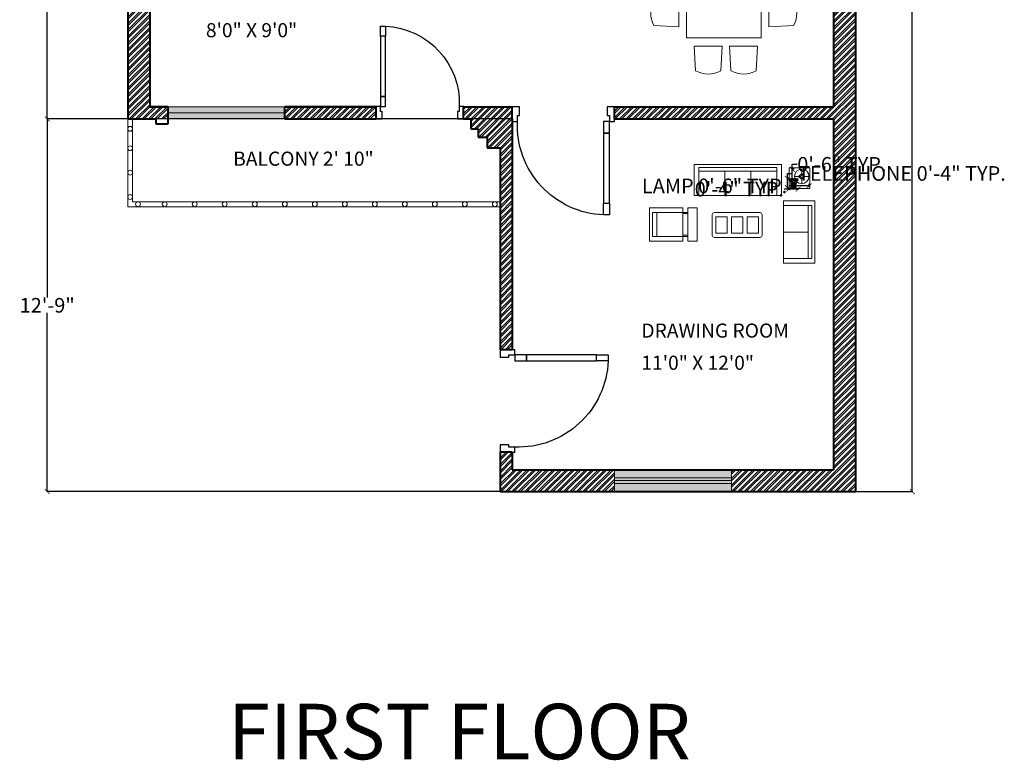
# Model space of a CAD drawing. Units: inches. Extents: x 528 to 2520, y -151 to 1354.
# Tile 15 of 41: x 1079 to 1484, y 706 to 1010. Entities that reach past the tile are written whole.
import ezdxf

# ---------------------------------------------------------------- set-up
doc = ezdxf.new("R2010")
doc.units = ezdxf.units.IN
doc.header["$MEASUREMENT"] = 0
for name, color, linetype, lineweight in [('A-ANNO-DIMS', 2, 'Continuous', 18), ('A-ANNO-TEXT', 7, 'Continuous', 30), ('A-AREA-IDEN', 7, 'Continuous', 18), ('A-Door', 150, 'Continuous', 25), ('A-FURN', 8, 'Continuous', 18), ('A-WALL-PATT', 6, 'Continuous', 13), ('KORKULUK', 4, 'Continuous', 20), ('walls', 7, 'Continuous', 40), ('WINDOWS', 2, 'Continuous', 20)]:
    doc.layers.add(name, color=color, linetype=linetype, lineweight=lineweight)
doc.layers.add('A-GLAZ-PATT', color=152, linetype='Continuous', lineweight=13, true_color=0x2776bb)
doc.layers.add('NT', color=1, linetype='Continuous')
doc.styles.get("Standard").update_dxf_attribs({"font": 'arial.ttf'})
doc.dimstyles.get("Standard").update_dxf_attribs({"dimtxt": 6, "dimasz": 2, "dimexe": 0.18, "dimexo": 0.0625, "dimgap": 0.09, "dimtad": 0, "dimtih": 1, "dimtoh": 1, "dimdec": 1, "dimzin": 0, "dimdsep": 46, "dimlunit": 3, "dimtxsty": 'Standard', "dimblk": 'ARCHTICK', "dimcen": 0.09, "dimadec": 0, "dimazin": 0, "dimtfac": 1, "dimtdec": 1, "dimtofl": 0, "dimtmove": 0, "dimatfit": 3, "dimfxl": 1, "dimtolj": 1, "dimtzin": 0, "dimarcsym": 0})

# ---------------------------------------------------------------- blocks, each defined once
blk = doc.blocks.new('A$C7DB75F4D')
at = {"layer": 'A-Door'}
for points in [[(625, 740), (625, 660), (665, 660), (665, 740)], [(625, 180), (625, 660), (665, 660), (665, 180)], [(625, 100), (625, 180), (665, 180), (665, 100)], [(35, 100), (35, 60), (50, 60), (50, 50), (50, 0), (0, 0), (0, 100)], [(665, 100), (700, 100), (700, 0), (650, 0), (650, 50), (650, 60), (665, 60)]]:
    blk.add_lwpolyline(points, close=True, dxfattribs=at)
at = {"layer": 'NT'}
blk.add_arc((650, 125), 615.5, 92.32782, 182.32782, dxfattribs=at)
blk = doc.blocks.new('RECLIN32')
for p, q in [((16, 0), (16, -32)), ((-11.5, -3), (11.5, -3)), ((-11.5, -32), (-11.5, -3)), ((-11.5, -7), (11.5, -7)), ((11.5, -3), (11.5, -32)), ((-11.5, -32), (-11.5, -37)), ((-10.5, -32), (-10.5, -37)), ((10.5, -32), (10.5, -37)), ((11.5, -32), (11.5, -37))]:
    blk.add_line(p, q)
blk.add_lwpolyline([(16, -32), (-16, -32), (-16, 0), (16, 0)])
blk.add_lwpolyline([(-16, -46), (-16, -37), (16, -37), (16, -46)], close=True)
blk = doc.blocks.new('LOVESET5')
for p, q in [((35.75, 0), (35.75, -30.00001)), ((-19.75, -3), (31.25, -3)), ((-19.75, -30.00001), (-19.75, -3)), ((-19.75, -6.5), (31.25, -6.5)), ((5.75, -6.5), (5.75, -30.00001)), ((31.25, -3), (31.25, -30.00001))]:
    blk.add_line(p, q)
for points in [[(35.75, -30.00001), (-24.25, -30.00001), (-24.25, 0), (24.25, 0)], [(24.25, 0), (35.75, 0)]]:
    blk.add_lwpolyline(points)
blk = doc.blocks.new('TBLEN20S')
blk.add_lwpolyline([(-10, -10), (-10, 10), (10, 10), (10, -10)], close=True)
blk = doc.blocks.new('LAMP')
for p, q in [((-1, 0), (-7, 0)), ((0, 3), (-3, 0)), ((-3, 0), (0, -3)), ((0, 7), (0, 1)), ((3, 0), (0, 3)), ((0, -3), (3, 0)), ((1, 0), (7, 0)), ((0, -1), (0, -7))]:
    blk.add_line(p, q)
for radius in [7, 1]:
    blk.add_circle((0, 0), radius)
blk = doc.blocks.new('SOFA7')
for p, q in [((-37.5, -3), (37.5, -3)), ((-37.5, -30), (-37.5, -3)), ((-37.5, -6.5), (37.5, -6.5)), ((-12.5, -6.5), (-12.5, -30)), ((12.5, -6.5), (12.5, -30)), ((37.5, -3), (37.5, -30))]:
    blk.add_line(p, q)
blk.add_lwpolyline([(-42, -30), (-42, 0), (42, 0), (42, -30)], close=True)
blk = doc.blocks.new('TBLWGLAS')
for p, q in [((-22, 0), (22, 0)), ((-24, -22), (-24, -2)), ((-20.5, -20), (-20.5, -4)), ((-20.5, -4), (-9.5, -4)), ((-9.5, -4), (-9.5, -20)), ((-5.5, -20), (-5.5, -4)), ((-5.5, -4), (5.5, -4)), ((5.5, -4), (5.5, -20)), ((9.5, -20), (9.5, -4)), ((9.5, -4), (20.5, -4)), ((20.5, -4), (20.5, -20)), ((24, -2), (24, -22)), ((22, -24), (-22, -24)), ((-9.5, -20), (-20.5, -20)), ((5.5, -20), (-5.5, -20)), ((20.5, -20), (9.5, -20))]:
    blk.add_line(p, q)
for centre, start, end in [((-22, -2), 90, 180), ((22, -2), 0, 90), ((-22, -22), 180, 270), ((22, -22), 270, 0)]:
    blk.add_arc(centre, 2, start, end)
blk = doc.blocks.new('PHONE')
for p, q in [((-3.99, 3.5), (-3.99, 2.5)), ((4.01, 3.5), (-3.99, 3.5)), ((-3.99, 2.5), (4.01, 2.5)), ((-2.49, -4.03), (-2.49, 1.92)), ((-2.02, 4.5), (2.02, 4.5)), ((-1.99, 1), (-1.99, -4)), ((2.01, 1), (-1.99, 1)), ((-1.49, 4), (-0.74, 4)), ((-1.49, 3.5), (-1.49, 4)), ((-1.49, 2), (-1.49, 2.5)), ((-0.74, 2), (-1.49, 2)), ((1.01, 0.5), (-0.99, 0.5)), ((-0.99, 0.5), (-0.99, -3.5)), ((-0.74, 4), (-0.74, 3.5)), ((-0.74, 2.5), (-0.74, 2)), ((0.76, 4), (0.76, 3.5)), ((1.51, 4), (0.76, 4)), ((0.76, 2.5), (0.76, 2)), ((0.76, 2), (1.51, 2)), ((1.01, -3.5), (1.01, 0.5)), ((1.51, 3.5), (1.51, 4)), ((1.51, 2), (1.51, 2.5)), ((2.01, -4), (2.01, 1)), ((2.51, 1.95), (2.51, -4.06)), ((4.01, 2.5), (4.01, 3.5)), ((2.04, -4.5), (-2.01, -4.5)), ((-1.99, -4), (2.01, -4)), ((-0.99, -3.5), (1.01, -3.5))]:
    blk.add_line(p, q)
for centre, radius, start, end in [((-3.24, 3), 1.27, 24.02748, 336.6167), ((-2.05, 4.06), 0.442, 81.8699, 188.1301), ((2.07, 4.06), 0.442, 351.8699, 98.1301), ((3.26, 3), 1.25, 205.0096, 154.8206), ((-2.05, -4.06), 0.442, 171.8699, 278.1301), ((2.07, -4.06), 0.442, 261.8699, 8.1301)]:
    blk.add_arc(centre, radius, start, end)
blk = doc.blocks.new('table-20')
at = {"color": 0, "linetype": 'ByBlock'}
for p, q in [((-1.052, 0.533), (-1.074, 0.134)), ((-0.646, 0.533), (-0.624, 0.134)), ((-0.484, 0.533), (-0.506, 0.134)), ((-0.078, 0.533), (-0.056, 0.134)), ((-1.2, 0), (0, 0)), ((-1.2, -0.8), (-1.2, 0)), ((-0.624, 0.134), (-1.074, 0.134)), ((-0.056, 0.134), (-0.506, 0.134)), ((0, -0.8), (0, 0)), ((-1.723, -0.197), (-1.324, -0.175)), ((-1.324, -0.625), (-1.324, -0.175)), ((0.124, -0.625), (0.124, -0.175)), ((0.523, -0.197), (0.124, -0.175)), ((-1.723, -0.603), (-1.324, -0.625)), ((0.523, -0.603), (0.124, -0.625)), ((-1.2, -0.8), (0, -0.8)), ((-0.624, -0.934), (-1.074, -0.934)), ((-1.052, -1.333), (-1.074, -0.934)), ((-0.646, -1.333), (-0.624, -0.934)), ((-0.484, -1.333), (-0.506, -0.934)), ((-0.056, -0.934), (-0.506, -0.934)), ((-0.078, -1.333), (-0.056, -0.934))]:
    blk.add_line(p, q, dxfattribs=at)
for centre, start, end in [((-0.849, 0.159), 61.4891, 118.5109), ((-0.281, 0.159), 61.4891, 118.5109), ((-1.349, -0.4), 151.4891, 208.5109), ((0.149, -0.4), 331.4891, 28.5109), ((-0.849, -0.959), 241.4891, 298.5109), ((-0.281, -0.959), 241.4891, 298.5109)]:
    blk.add_arc(centre, 0.425, start, end, dxfattribs=at)
blk = doc.blocks.new('_ArchTick')
at = {"color": 0, "linetype": 'ByBlock', "const_width": 0.15}
blk.add_lwpolyline([(-0.5, -0.5), (0.5, 0.5)], dxfattribs=at)
blk = doc.blocks.new('*D26')
at = {"layer": 'A-ANNO-DIMS', "color": 0, "lineweight": -2, "transparency": 16777216}
for p, q in [((1422.95, 1317.1), (1446.41, 1317.1)), ((1446.23, 1317.1), (1446.23, 1069.76)), ((1446.23, 816.1), (1446.23, 1063.45)), ((1422.95, 816.1), (1446.41, 816.1))]:
    blk.add_line(p, q, dxfattribs=at)
at = {"layer": 'Defpoints', "color": 0, "transparency": 16777216}
for p in [(1422.88, 1317.1), (1422.88, 816.1), (1446.23, 816.1)]:
    blk.add_point(p, dxfattribs=at)
at = {"layer": 'A-ANNO-DIMS', "color": 0, "lineweight": -2, "transparency": 16777216, "xscale": 2, "yscale": 2, "zscale": 2}
for p, rotation in [((1446.23, 1317.1), 90), ((1446.23, 816.1), 270)]:
    blk.add_blockref('_ArchTick', p, dxfattribs=dict(at, rotation=rotation))
at = {"layer": 'A-ANNO-DIMS', "color": 0, "transparency": 16777216, "insert": (1446.23, 1066.6), "char_height": 6, "attachment_point": 5}
blk.add_mtext('\\A1;41\'-9.0"', dxfattribs=at)
blk = doc.blocks.new('WINDOW-48x5-PLAN')
for p, q in [((0, 5), (48, 5)), ((0, 2.5), (48, 2.5))]:
    blk.add_line(p, q)
blk.add_lwpolyline([(0, 5), (48, 5), (48, 0), (0, 0)], close=True)
blk = doc.blocks.new('WINDOW-48x9-PLAN')
for p, q in [((0, 5.63), (48, 5.63)), ((0, 4.5), (48, 4.5)), ((0, 3.37), (48, 3.37))]:
    blk.add_line(p, q)
blk.add_lwpolyline([(0, 9), (48, 9), (48, 0), (0, 0)], close=True)
blk = doc.blocks.new('TELEPHONE-KEYPAD')
for centre in [(0.05, 0.67), (0.07, 0.46), (0.09, 0.25), (0.1, 0.06), (0.26, 0.67), (0.27, 0.47), (0.27, 0.25), (0.29, 0.05), (0.48, 0.66), (0.48, 0.46), (0.49, 0.26), (0.5, 0.08)]:
    blk.add_circle(centre, 0.0493)
blk = doc.blocks.new('*D68')
at = {"layer": 'A-ANNO-DIMS', "color": 0, "lineweight": -2, "transparency": 16777216}
for p, q in [((1397.81, 941.62), (1395.81, 941.62)), ((1397.81, 942.45), (1397.81, 941.44)), ((1403.79, 941.62), (1397.81, 941.62)), ((1403.79, 942.45), (1403.79, 941.44))]:
    blk.add_line(p, q, dxfattribs=at)
at = {"layer": 'Defpoints', "color": 0, "transparency": 16777216}
for p in [(1397.81, 942.52), (1397.81, 941.62), (1403.79, 942.52)]:
    blk.add_point(p, dxfattribs=at)
at = {"layer": 'A-ANNO-DIMS', "color": 0, "lineweight": -2, "transparency": 16777216, "xscale": 2, "yscale": 2, "zscale": 2, "rotation": 180}
blk.add_blockref('_ArchTick', (1397.81, 941.62), dxfattribs=at)
at = {"layer": 'A-ANNO-DIMS', "color": 0, "lineweight": -2, "transparency": 16777216, "xscale": 2, "yscale": 2, "zscale": 2}
blk.add_blockref('_ArchTick', (1403.79, 941.62), dxfattribs=at)
at = {"layer": 'A-ANNO-DIMS', "color": 0, "transparency": 16777216, "insert": (1364.99, 941.62), "char_height": 6, "attachment_point": 5}
blk.add_mtext('\\A1;LAMP 0\'-6" TYP.', dxfattribs=at)
blk = doc.blocks.new('*D69')
at = {"layer": 'A-ANNO-DIMS', "color": 0, "lineweight": -2, "transparency": 16777216}
for p, q in [((1397.75, 948.49), (1396.74, 948.49)), ((1396.92, 948.49), (1396.92, 950.49)), ((1396.92, 950.49), (1398.92, 950.49)), ((1396.92, 942.52), (1396.92, 948.49)), ((1397.75, 942.52), (1396.74, 942.52))]:
    blk.add_line(p, q, dxfattribs=at)
at = {"layer": 'Defpoints', "color": 0, "transparency": 16777216}
for p in [(1396.92, 948.49), (1397.81, 948.49), (1397.81, 942.52)]:
    blk.add_point(p, dxfattribs=at)
at = {"layer": 'A-ANNO-DIMS', "color": 0, "lineweight": -2, "transparency": 16777216, "xscale": 2, "yscale": 2, "zscale": 2}
for p, rotation in [((1396.92, 948.49), 90), ((1396.92, 942.52), 270)]:
    blk.add_blockref('_ArchTick', p, dxfattribs=dict(at, rotation=rotation))
at = {"layer": 'A-ANNO-DIMS', "color": 0, "transparency": 16777216, "insert": (1417.29, 950.49), "char_height": 6, "attachment_point": 5}
blk.add_mtext('\\A1;0\'-6" TYP.', dxfattribs=at)
blk = doc.blocks.new('*D74')
at = {"layer": 'A-ANNO-DIMS', "color": 0, "lineweight": -2, "transparency": 16777216}
for p, q in [((1394.94, 944.74), (1394.94, 946.74)), ((1394.94, 946.74), (1396.94, 946.74)), ((1395.45, 944.74), (1394.76, 944.74)), ((1394.94, 940.88), (1394.94, 944.74)), ((1395.45, 940.88), (1394.76, 940.88))]:
    blk.add_line(p, q, dxfattribs=at)
at = {"layer": 'Defpoints', "color": 0, "transparency": 16777216}
for p in [(1394.94, 944.74), (1395.52, 944.74), (1395.52, 940.88)]:
    blk.add_point(p, dxfattribs=at)
at = {"layer": 'A-ANNO-DIMS', "color": 0, "lineweight": -2, "transparency": 16777216, "xscale": 2, "yscale": 2, "zscale": 2}
for p, rotation in [((1394.94, 944.74), 90), ((1394.94, 940.88), 270)]:
    blk.add_blockref('_ArchTick', p, dxfattribs=dict(at, rotation=rotation))
at = {"layer": 'A-ANNO-DIMS', "color": 0, "transparency": 16777216, "insert": (1441.94, 946.74), "char_height": 6, "attachment_point": 5}
blk.add_mtext('\\A1;TELEPHONE 0\'-4" TYP.', dxfattribs=at)
blk = doc.blocks.new('*D75')
at = {"layer": 'A-ANNO-DIMS', "color": 0, "lineweight": -2, "transparency": 16777216}
for p, q in [((1395.52, 940.3), (1393.52, 940.3)), ((1395.52, 940.82), (1395.52, 940.12)), ((1399.37, 940.3), (1395.52, 940.3)), ((1399.37, 940.82), (1399.37, 940.12))]:
    blk.add_line(p, q, dxfattribs=at)
at = {"layer": 'Defpoints', "color": 0, "transparency": 16777216}
for p in [(1395.52, 940.88), (1395.52, 940.3), (1399.37, 940.88)]:
    blk.add_point(p, dxfattribs=at)
at = {"layer": 'A-ANNO-DIMS', "color": 0, "lineweight": -2, "transparency": 16777216, "xscale": 2, "yscale": 2, "zscale": 2, "rotation": 180}
blk.add_blockref('_ArchTick', (1395.52, 940.3), dxfattribs=at)
at = {"layer": 'A-ANNO-DIMS', "color": 0, "lineweight": -2, "transparency": 16777216, "xscale": 2, "yscale": 2, "zscale": 2}
blk.add_blockref('_ArchTick', (1399.37, 940.3), dxfattribs=at)
at = {"layer": 'A-ANNO-DIMS', "color": 0, "transparency": 16777216, "insert": (1375.14, 940.3), "char_height": 6, "attachment_point": 5}
blk.add_mtext('\\A1;0\'-4" TYP.', dxfattribs=at)
blk = doc.blocks.new('*D96')
at = {"layer": 'A-ANNO-DIMS', "color": 0, "lineweight": -2, "transparency": 16777216}
for p, q in [((1281.82, 969.1), (1090.6, 969.1)), ((1090.78, 969.1), (1090.78, 895.76)), ((1090.78, 816.1), (1090.78, 889.45)), ((1276.82, 816.1), (1090.6, 816.1))]:
    blk.add_line(p, q, dxfattribs=at)
at = {"layer": 'Defpoints', "color": 0, "transparency": 16777216}
for p in [(1090.78, 969.1), (1281.88, 969.1), (1276.88, 816.1)]:
    blk.add_point(p, dxfattribs=at)
at = {"layer": 'A-ANNO-DIMS', "color": 0, "lineweight": -2, "transparency": 16777216, "xscale": 2, "yscale": 2, "zscale": 2}
for p, rotation in [((1090.78, 969.1), 90), ((1090.78, 816.1), 270)]:
    blk.add_blockref('_ArchTick', p, dxfattribs=dict(at, rotation=rotation))
at = {"layer": 'A-ANNO-DIMS', "color": 0, "transparency": 16777216, "insert": (1090.78, 892.6), "char_height": 6, "attachment_point": 5}
blk.add_mtext('\\A1;12\'-9"', dxfattribs=at)
blk = doc.blocks.new('*D97')
at = {"layer": 'A-ANNO-DIMS', "color": 0, "lineweight": -2, "transparency": 16777216}
for p, q in [((1132.82, 1082.1), (1090.6, 1082.1)), ((1090.78, 1082.1), (1090.78, 1028.76)), ((1090.78, 969.1), (1090.78, 1022.45)), ((1123.82, 969.1), (1090.6, 969.1))]:
    blk.add_line(p, q, dxfattribs=at)
at = {"layer": 'Defpoints', "color": 0, "transparency": 16777216}
for p in [(1090.78, 1082.1), (1132.88, 1082.1), (1123.88, 969.1)]:
    blk.add_point(p, dxfattribs=at)
at = {"layer": 'A-ANNO-DIMS', "color": 0, "lineweight": -2, "transparency": 16777216, "xscale": 2, "yscale": 2, "zscale": 2}
for p, rotation in [((1090.78, 1082.1), 90), ((1090.78, 969.1), 270)]:
    blk.add_blockref('_ArchTick', p, dxfattribs=dict(at, rotation=rotation))
at = {"layer": 'A-ANNO-DIMS', "color": 0, "transparency": 16777216, "insert": (1090.78, 1025.6), "char_height": 6, "attachment_point": 5}
blk.add_mtext('\\A1;9\'-5"', dxfattribs=at)

msp = doc.modelspace()

# ---------------------------------------------------------------- hatches: boundary and pattern name
at = {"layer": 'A-GLAZ-PATT'}
h = msp.add_hatch(color=256, dxfattribs=at)
h.dxf.hatch_style = 1
h.paths.add_polyline_path([(1188.43, 974.1), (1140.43, 974.1), (1140.43, 971.6), (1188.43, 971.6)])
h.paths.add_polyline_path([(1188.43, 971.6), (1140.43, 971.6), (1140.43, 969.1), (1188.43, 969.1)])
h = msp.add_hatch(color=256, dxfattribs=at)
h.dxf.hatch_style = 1
h.paths.add_polyline_path([(1371.88, 825.1), (1323.88, 825.1), (1323.88, 821.73), (1371.88, 821.73)])
h.paths.add_polyline_path([(1371.88, 821.73), (1323.88, 821.73), (1323.88, 820.6), (1371.88, 820.6)])
h.paths.add_polyline_path([(1371.88, 820.6), (1323.88, 820.6), (1323.88, 819.47), (1371.88, 819.47)])
h.paths.add_polyline_path([(1371.88, 819.47), (1323.88, 819.47), (1323.88, 816.1), (1371.88, 816.1)])
at = {"layer": 'A-WALL-PATT'}
h = msp.add_hatch(dxfattribs=at)
h.set_pattern_fill('ANSI32', color=256, scale=5)
h.set_pattern_definition([(45, (537.1868, 0), (-1.3258252, 1.3258252), []), (45, (538.0707, 0), (-1.3258252, 1.3258252), [])])
h.paths.add_polyline_path([(1132.88, 1163.86), (1123.88, 1163.86), (1123.88, 969.1), (1135.43, 969.1), (1140.43, 969.1), (1140.43, 974.1), (1132.88, 974.1), (1132.88, 1082.1), (1228.88, 1082.1), (1228.88, 1087.1), (1228.88, 1106.1), (1234.88, 1106.1), (1234.88, 1111.1), (1223.88, 1111.1), (1223.88, 1087.1), (1132.88, 1087.1)])
h.paths.add_polyline_path([(1225.89, 974.1), (1188.43, 974.1), (1188.43, 969.1), (1225.89, 969.1)])
h.paths.add_polyline_path([(1422.88, 1171.37), (1413.88, 1171.37), (1413.88, 1111.1), (1323.88, 1111.1), (1323.88, 1106.1), (1413.88, 1106.1), (1413.88, 974.1), (1323.88, 974.1), (1323.88, 969.1), (1413.88, 969.1), (1413.88, 825.1), (1371.88, 825.1), (1371.88, 816.1), (1422.88, 816.1)])
h.paths.add_polyline_path([(1422.88, 1317.1), (1413.84, 1317.1), (1413.84, 1308.1), (1413.88, 1308.1), (1413.88, 1248.1), (1359.88, 1248.1), (1359.88, 1243.1), (1413.88, 1243.1), (1413.88, 1219.37), (1422.88, 1219.37)])
h.paths.add_polyline_path([(1389.84, 1317.1), (1324.88, 1317.1), (1324.88, 1248.1), (1321.45, 1248.1), (1321.45, 1243.1), (1329.88, 1243.1), (1329.88, 1249.1), (1329.88, 1308.1), (1389.84, 1308.1)])
h.paths.add_polyline_path([(1221.88, 1317.1), (1156.88, 1317.1), (1156.88, 1308.1), (1216.88, 1308.1), (1216.88, 1248.1), (1216.88, 1243.1), (1221.88, 1243.1), (1221.88, 1248.25)])
h.paths.add_polyline_path([(1132.88, 1308.1), (1132.88, 1317.1), (1123.88, 1317.1), (1123.88, 1211.86), (1132.88, 1211.86), (1132.88, 1243.1), (1186.88, 1243.1), (1186.88, 1248.1), (1132.88, 1248.1)])
h.paths.add_polyline_path([(1281.88, 969.1), (1281.88, 974.1), (1261.89, 974.1), (1261.89, 969.1), (1276.88, 969.1), (1276.88, 874.29), (1281.88, 874.29)])
h.paths.add_polyline_path([(1276.88, 969.1), (1264.88, 969.1), (1264.88, 965.12), (1267.92, 965.12), (1267.92, 961.68), (1271.62, 961.68), (1271.62, 957.24), (1276.88, 957.24)], flags=17)
h.paths.add_polyline_path([(1323.88, 825.1), (1281.88, 825.1), (1281.88, 832.29), (1276.88, 832.29), (1276.88, 816.1), (1323.88, 816.1)])

# ---------------------------------------------------------------- linework, layer by layer
at = {"layer": 'KORKULUK'}
for p, q in [((1123.88, 969.1), (1123.88, 933.1)), ((1125.88, 969.1), (1125.88, 935.1)), ((1125.88, 935.1), (1276.88, 935.1)), ((1123.88, 933.1), (1276.88, 933.1))]:
    msp.add_line(p, q, dxfattribs=at)
for centre in [(1124.88, 965.06), (1124.88, 957.08), (1124.88, 947.08), (1124.88, 937.08), (1128.07, 934.1), (1139.07, 934.1), (1151.4, 934.1), (1163.73, 934.1), (1176.06, 934.1), (1188.39, 934.1), (1200.72, 934.1), (1213.05, 934.1), (1225.38, 934.1), (1237.71, 934.1), (1250.04, 934.1), (1262.37, 934.1), (1274.7, 934.1)]:
    msp.add_circle(centre, 1, dxfattribs=at)
at = {"layer": 'walls'}
for p, q in [((1123.88, 1317.1), (1123.88, 969.1)), ((1422.88, 1317.1), (1422.88, 816.1)), ((1413.88, 1106.1), (1413.88, 974.1)), ((1132.88, 1082.1), (1132.88, 974.1)), ((1132.88, 974.1), (1140.43, 974.1)), ((1140.43, 974.1), (1132.88, 974.1)), ((1140.43, 967.1), (1140.43, 974.1)), ((1188.43, 974.1), (1225.89, 974.1)), ((1225.89, 974.1), (1188.43, 974.1)), ((1188.43, 969.1), (1188.43, 974.1)), ((1225.89, 969.1), (1225.89, 974.1)), ((1261.89, 974.1), (1281.88, 974.1)), ((1261.89, 969.1), (1261.89, 974.1)), ((1281.88, 969.1), (1281.88, 974.1)), ((1323.88, 974.1), (1413.88, 974.1)), ((1323.88, 969.1), (1323.88, 974.1)), ((1123.88, 969.1), (1135.43, 969.1)), ((1135.43, 969.1), (1135.43, 967.1)), ((1135.43, 967.1), (1140.43, 967.1)), ((1188.43, 969.1), (1225.89, 969.1)), ((1261.89, 969.1), (1264.88, 969.1)), ((1264.88, 969.1), (1264.88, 965.12)), ((1281.88, 969.1), (1281.88, 874.29)), ((1323.88, 969.1), (1413.88, 969.1)), ((1413.88, 969.1), (1413.88, 825.1)), ((1264.88, 965.12), (1267.92, 965.12)), ((1267.92, 965.12), (1267.92, 961.68)), ((1267.92, 961.68), (1271.62, 961.68)), ((1271.62, 961.68), (1271.62, 957.24)), ((1271.62, 957.24), (1276.88, 957.24)), ((1276.88, 957.24), (1276.88, 874.29)), ((1281.88, 874.29), (1276.88, 874.29)), ((1276.88, 832.29), (1276.88, 816.1)), ((1281.88, 832.29), (1276.88, 832.29)), ((1281.88, 832.29), (1281.88, 825.1)), ((1281.88, 825.1), (1413.88, 825.1)), ((1276.88, 816.1), (1422.88, 816.1))]:
    msp.add_line(p, q, dxfattribs=at)

# ---------------------------------------------------------------- block references
at = {"layer": 'A-Door', "xscale": -0.0514539602427209, "yscale": 0.0514539602427209, "zscale": 0.0514539602427209}
msp.add_blockref('A$C7DB75F4D', (1261.91, 969.1), dxfattribs=at)
at = {"layer": 'A-Door', "xscale": -0.0600000000000059, "yscale": 0.0600000000000059, "zscale": 0.0600000000000059}
for p, rotation in [((1281.88, 974.1), 180), ((1276.88, 832.29), 270)]:
    msp.add_blockref('A$C7DB75F4D', p, dxfattribs=dict(at, rotation=rotation))
at = {"layer": 'A-FURN', "xscale": 25.57841077690889, "yscale": 25.57841077690889, "zscale": 25.57841077690889}
msp.add_blockref('table-20', (1384.12, 1022.96), dxfattribs=at)
at = {"layer": 'A-FURN', "extrusion": (0, 0, -1), "xscale": 0.4266539259093383, "yscale": 0.4266539259093383, "zscale": -0.426653925909338}
for name, p in [('SOFA7', (-1374.52, 950.48)), ('TBLEN20S', (-1399.85, 944.79)), ('LAMP', (-1400.8, 945.5)), ('PHONE', (-1397.44, 942.81)), ('TBLWGLAS', (-1374.28, 930.69))]:
    msp.add_blockref(name, p, dxfattribs=at)
at = {"layer": 'A-FURN'}
msp.add_blockref('TELEPHONE-KEYPAD', (1397.18, 942.09), dxfattribs=at)
at = {"layer": 'A-FURN', "extrusion": (0, 0, -1), "xscale": 0.4266539259093436, "yscale": 0.4266539259093436, "zscale": -0.426653925909338}
for name, p, rotation in [('LOVESET5', (-1406.17, 920.23), 89.99999999999947), ('RECLIN32', (-1338.23, 925.82), 269.9999999999994)]:
    msp.add_blockref(name, p, dxfattribs=dict(at, rotation=rotation))
at = {"layer": 'WINDOWS'}
for name, p in [('WINDOW-48x5-PLAN', (1140.43, 969.1)), ('WINDOW-48x9-PLAN', (1323.88, 816.1))]:
    msp.add_blockref(name, p, dxfattribs=at)

# ---------------------------------------------------------------- texts
at = {"layer": 'A-ANNO-TEXT'}
msp.add_text('FIRST FLOOR', height=22.7949, dxfattribs=at).set_placement((1165.1, 706.16))
at = {"layer": 'A-AREA-IDEN'}
for s, p in [('8\'0" X 9\'0"', (1155.99, 1002.67)), ('BALCONY 2\' 10"', (1167.19, 949.91)), ('DRAWING ROOM', (1334.92, 879.32)), ('11\'0" X 12\'0"', (1334.92, 866.1))]:
    msp.add_text(s, height=5.7926, dxfattribs=at).set_placement(p)

# ---------------------------------------------------------------- dimensions: what is measured, and where the dimension line sits
at = {"layer": 'A-ANNO-DIMS'}
for base, p1, p2, override, picture, middle in [((1446.23, 816.1), (1422.88, 1317.1), (1422.88, 816.1), {"dimclrd": 0, "dimclre": 0, "dimclrt": 0}, '*D26', (1446.23, 1066.6)), ((1090.78, 1082.1), (1123.88, 969.1), (1132.88, 1082.1), {"dimdec": 1, "dimlfac": 1, "dimrnd": 0, "dimzin": 1, "dimdsep": 46, "dimlunit": 4, "dimfrac": 2}, '*D97', (1090.78, 1025.6)), ((1090.78, 969.1), (1276.88, 816.1), (1281.88, 969.1), {"dimdec": 1, "dimlfac": 1, "dimrnd": 0, "dimzin": 1, "dimdsep": 46, "dimlunit": 4, "dimfrac": 2}, '*D96', (1090.78, 892.6))]:
    dim = msp.add_linear_dim(base=base, p1=p1, p2=p2, angle=90, dimstyle='Standard', override=override, dxfattribs=at)
    dim.commit()
    dim.dimension.update_dxf_attribs({"geometry": picture, "text_midpoint": middle})
for base, p1, p2, angle, text, picture, middle in [((1394.94, 944.74), (1395.52, 940.88), (1395.52, 944.74), 90, 'TELEPHONE <> TYP.', '*D74', (1441.94, 946.74)), ((1396.92, 948.49), (1397.81, 942.52), (1397.81, 948.49), 90, '<> TYP.', '*D69', (1417.29, 950.49)), ((1397.81, 941.62), (1403.79, 942.52), (1397.81, 942.52), 180, 'LAMP <> TYP.', '*D68', (1364.99, 941.62)), ((1395.5158, 940.3032), (1399.368, 940.8817), (1395.5158, 940.8817), 180, '<> TYP.', '*D75', (1375.1393, 940.3032))]:
    dim = msp.add_linear_dim(base=base, p1=p1, p2=p2, angle=angle, text=text, dimstyle='Standard', override={"dimdec": 1, "dimlfac": 1, "dimrnd": 0, "dimzin": 1, "dimdsep": 46, "dimlunit": 4, "dimfrac": 2}, dxfattribs=at)
    dim.commit()
    dim.dimension.update_dxf_attribs({"geometry": picture, "text_midpoint": middle})

doc.saveas('drawing.dxf')
